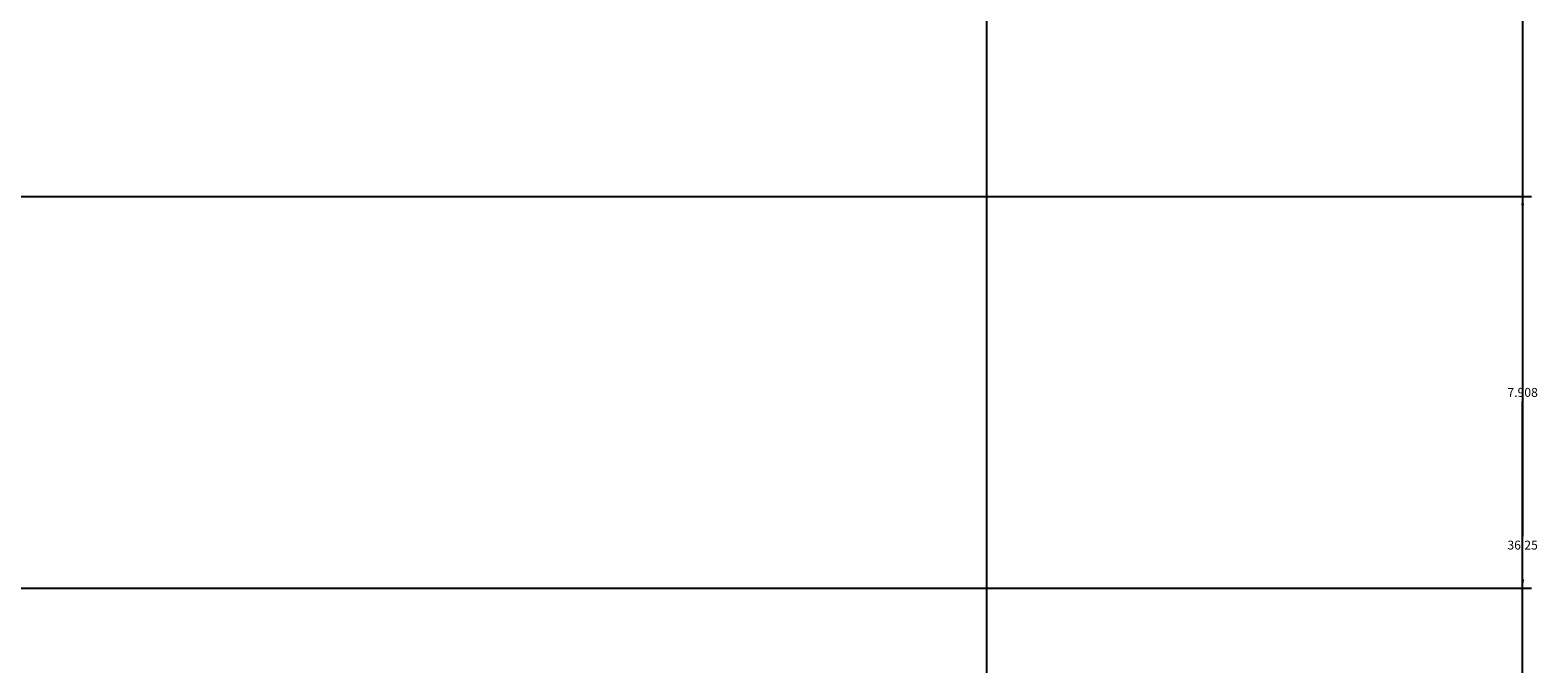
# Model space of a CAD drawing. Units: inches. Extents: x -117 to 121, y -77 to 40.
# Tile 42 of 45: x 91 to 121, y -23 to -10. Entities that reach past the tile are written whole.
import ezdxf

# ---------------------------------------------------------------- set-up
doc = ezdxf.new("R2010")
doc.units = ezdxf.units.IN
doc.header["$MEASUREMENT"] = 0
doc.layers.add('A-ANNO-DIMS', color=2, linetype='Continuous', lineweight=18)
doc.styles.get("Standard").update_dxf_attribs({"font": 'arial.ttf'})
doc.dimstyles.get("Standard").update_dxf_attribs({"dimtxt": 0.18, "dimasz": 0.18, "dimexe": 0.18, "dimexo": 0.0625, "dimgap": 0.09, "dimtad": 0, "dimtih": 1, "dimtoh": 1, "dimdec": 4, "dimzin": 0, "dimdsep": 46, "dimtxsty": 'Standard', "dimcen": 0.09, "dimadec": 0, "dimazin": 0, "dimtfac": 1, "dimtdec": 4, "dimtofl": 0, "dimtmove": 0, "dimatfit": 3, "dimfxl": 1, "dimtolj": 1, "dimtzin": 0, "dimarcsym": 0})

# ---------------------------------------------------------------- blocks, each defined once
blk = doc.blocks.new('*D15')
at = {"layer": 'A-ANNO-DIMS', "color": 0, "lineweight": -2, "transparency": 16777216}
for p, q in [((87.304, -2.653), (120.84, -2.653)), ((120.66, -2.833), (120.66, -20.595)), ((120.66, -38.722), (120.66, -20.959)), ((90.611, -38.902), (120.84, -38.902))]:
    blk.add_line(p, q, dxfattribs=at)
at = {"layer": 'A-ANNO-DIMS', "color": 0, "transparency": 16777216}
for points in [[(120.63, -2.833), (120.69, -2.833), (120.66, -2.653)], [(120.63, -38.722), (120.69, -38.722), (120.66, -38.902)]]:
    blk.add_solid(points, dxfattribs=at)
at = {"layer": 'Defpoints', "color": 0, "transparency": 16777216}
for p in [(87.242, -2.653), (90.549, -38.902), (120.66, -38.902)]:
    blk.add_point(p, dxfattribs=at)
at = {"layer": 'A-ANNO-DIMS', "color": 0, "transparency": 16777216, "insert": (120.66, -20.777), "char_height": 0.18, "attachment_point": 5}
blk.add_mtext('\\A1;36.25', dxfattribs=at)
blk = doc.blocks.new('*D24')
at = {"layer": 'A-ANNO-DIMS', "color": 0, "lineweight": -2, "transparency": 16777216}
for p, q in [((87.242, 3.166), (87.242, 38.61)), ((87.422, 38.43), (98.081, 38.43)), ((109.67, 38.43), (99.011, 38.43)), ((109.85, -61.313), (109.85, 38.61))]:
    blk.add_line(p, q, dxfattribs=at)
at = {"layer": 'A-ANNO-DIMS', "color": 0, "transparency": 16777216}
for points in [[(87.422, 38.46), (87.422, 38.4), (87.242, 38.43)], [(109.67, 38.46), (109.67, 38.4), (109.85, 38.43)]]:
    blk.add_solid(points, dxfattribs=at)
at = {"layer": 'Defpoints', "color": 0, "transparency": 16777216}
for p in [(109.85, 38.43), (87.242, 3.104), (109.85, -61.376)]:
    blk.add_point(p, dxfattribs=at)
at = {"layer": 'A-ANNO-DIMS', "color": 0, "transparency": 16777216, "insert": (98.546, 38.43), "char_height": 0.18, "attachment_point": 5}
blk.add_mtext('\\A1;22.609', dxfattribs=at)
blk = doc.blocks.new('*D50')
at = {"layer": 'A-ANNO-DIMS', "color": 0, "lineweight": -2, "transparency": 16777216}
for p, q in [((-47.458, -13.74), (120.84, -13.74)), ((120.66, -13.92), (120.66, -17.512)), ((120.66, -21.468), (120.66, -17.876)), ((-47.458, -21.648), (120.84, -21.648))]:
    blk.add_line(p, q, dxfattribs=at)
at = {"layer": 'A-ANNO-DIMS', "color": 0, "transparency": 16777216}
for points in [[(120.63, -13.92), (120.69, -13.92), (120.66, -13.74)], [(120.63, -21.468), (120.69, -21.468), (120.66, -21.648)]]:
    blk.add_solid(points, dxfattribs=at)
at = {"layer": 'Defpoints', "color": 0, "transparency": 16777216}
for p in [(-47.521, -13.74), (120.66, -13.74), (-47.521, -21.648)]:
    blk.add_point(p, dxfattribs=at)
at = {"layer": 'A-ANNO-DIMS', "color": 0, "transparency": 16777216, "insert": (120.66, -17.694), "char_height": 0.18, "attachment_point": 5}
blk.add_mtext('\\A1;7.908', dxfattribs=at)

msp = doc.modelspace()

# ---------------------------------------------------------------- dimensions: what is measured, and where the dimension line sits
at = {"layer": 'A-ANNO-DIMS'}
dim = msp.add_linear_dim(base=(109.8502, 38.4297), p1=(87.2416, 3.1036), p2=(109.8502, -61.3756), dimstyle='Standard', override={"dimdec": 3, "dimlfac": 1, "dimrnd": 0, "dimzin": 0, "dimdsep": 46, "dimlunit": 2}, dxfattribs=at)
dim.commit()
dim.dimension.update_dxf_attribs({"geometry": '*D24', "text_midpoint": (98.5459, 38.4297)})
for base, p1, p2, override, picture, middle in [((120.6602, -38.9022), (87.2416, -2.6528), (90.5486, -38.9022), {"dimdec": 2, "dimlfac": 1, "dimrnd": 0, "dimzin": 0, "dimdsep": 46, "dimlunit": 2}, '*D15', (120.6602, -20.7775)), ((120.6602, -13.74), (-47.5206, -21.6476), (-47.5206, -13.74), {"dimdec": 3, "dimlfac": 1, "dimrnd": 0, "dimzin": 0, "dimdsep": 46, "dimlunit": 2}, '*D50', (120.6602, -17.6938))]:
    dim = msp.add_linear_dim(base=base, p1=p1, p2=p2, angle=90, dimstyle='Standard', override=override, dxfattribs=at)
    dim.commit()
    dim.dimension.update_dxf_attribs({"geometry": picture, "text_midpoint": middle})

doc.saveas('drawing.dxf')
